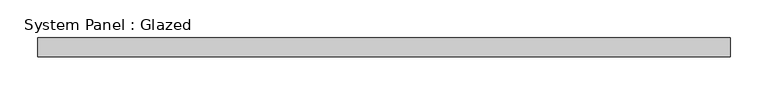
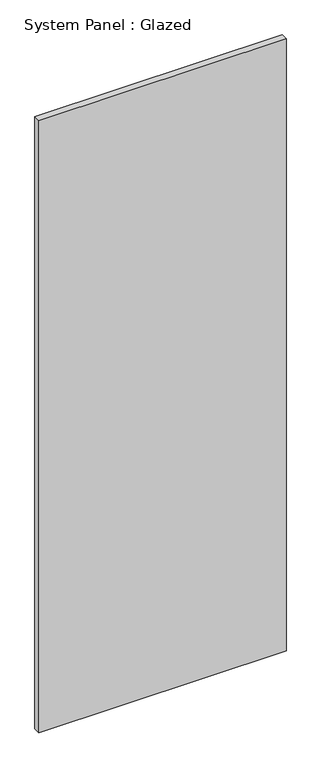
"""IFC4 building model written with IfcOpenShell, lengths in millimetres: plate geometry, System Panel : Glazed."""

from ifc_helpers import new_model, si_unit, origin, origin_with_axes, place, context, project, spatial, polyline, outline, extrude, source, transform, mapped, element, save


def system_panel_glazed_5062b81b(model_context):
    return source(origin(), model_context, "Body", "SweptSolid", [
        extrude(outline(polyline([(460.375, 19.05), (-460.375, 19.05), (-460.375, 44.45), (460.375, 44.45), (460.375, 19.05)])), origin_with_axes(), (0.0, 0.0, 1.0), 2411.6388159),
    ])


if __name__ == "__main__":
    model = new_model("IFC4")
    model_context = context("Model", 3, world=origin())
    ifc_project = project(units=[si_unit("LENGTHUNIT", "METRE", prefix="MILLI")], contexts=[model_context])
    site = spatial("IfcSite", under=ifc_project)
    building = spatial("IfcBuilding", under=site)
    placement = place(None, origin())
    system_panel_glazed_shape = system_panel_glazed_5062b81b(model_context)
    element("IfcPlate", 1, ObjectType="System Panel : Glazed", at=placement, inside=building, context=model_context, shape_type="MappedRepresentation", body=[
        mapped(system_panel_glazed_shape, transform((0.0, 0.0, 0.0), x_axis=(1.0, 0.0, 0.0), y_axis=(0.0, 1.0, 0.0), z_axis=(0.0, 0.0, 1.0))),
    ])
    save(model, "model.ifc")

# Revit data of these elements
# Type "System Panel : Glazed"
#   Construction Type Id = "GSP4R"
#   Analytic Construction = "1/8 in Pilkington single glazing"
#   Visual Light Transmittance = 0.9
#   Solar Heat Gain Coefficient = 0.86
#   Heat Transfer Coefficient (U) = 1.18115 BTU/(h·ft²·°F)
#   Define Thermal Properties by = 1
# Element 1 (IfcPlate, "System Panel : Glazed")
#   Materials on its faces: "Glass"
# Materials
#   "Glass": class "Glass", colour RGB 0 128 192, transparency 0.75, Description = "Soda Lime Glass", Cost = 0
